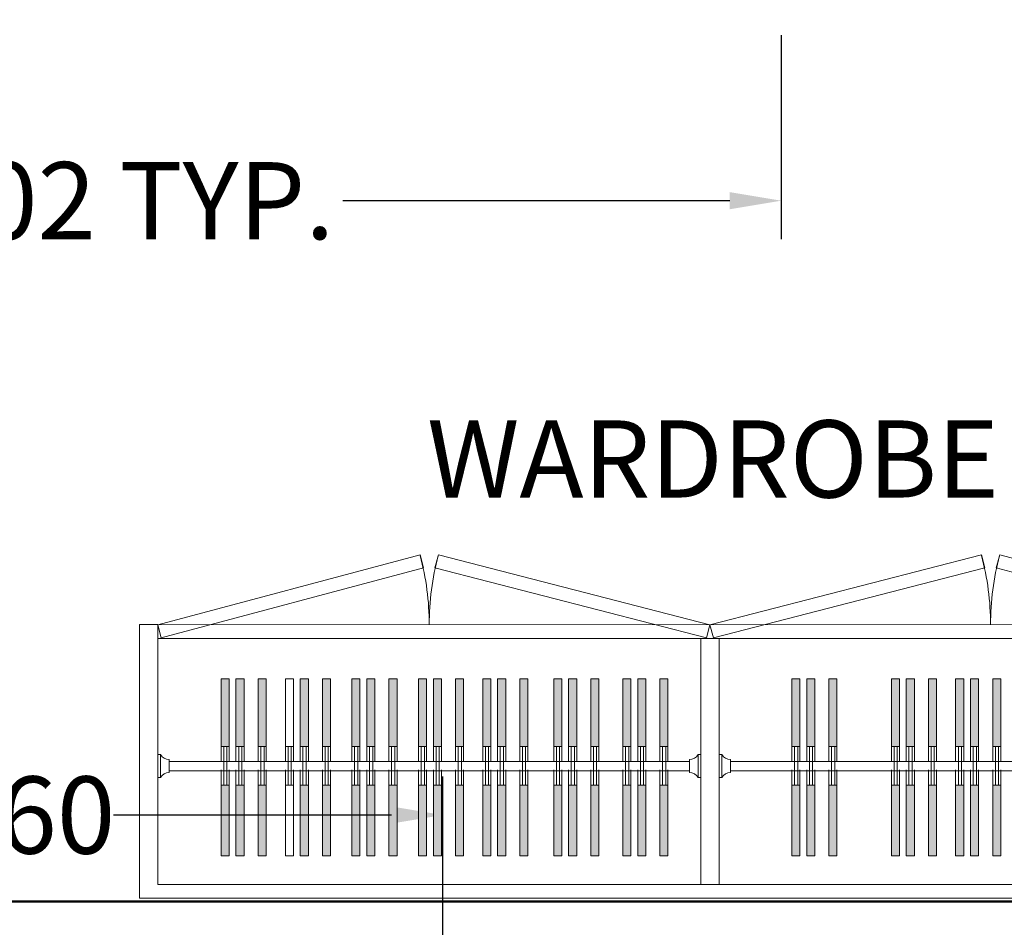
# Model space of a CAD drawing. Units: inches. Extents: x -466983 to 1020, y 324 to 318697.
# Tile 94 of 97: x 864 to 940, y 827 to 898. Entities that reach past the tile are written whole.
import ezdxf

# ---------------------------------------------------------------- set-up
doc = ezdxf.new("R2010")
doc.units = ezdxf.units.IN
doc.header["$MEASUREMENT"] = 0
for name, color, linetype, lineweight in [('A-ANNO-DIMS', 2, 'Continuous', 18), ('A-ANNO-TEXT', 7, 'Continuous', 18), ('A-FLOR-PATT', 252, 'Continuous', 13), ('A-FURN', 8, 'Continuous', 18), ('A-WALL', 7, 'Continuous', 50)]:
    doc.layers.add(name, color=color, linetype=linetype, lineweight=lineweight)
doc.styles.get("Standard").update_dxf_attribs({"font": 'arial.ttf'})
doc.dimstyles.get("Standard").update_dxf_attribs({"dimtxt": 6, "dimasz": 4, "dimexe": 3, "dimexo": 3, "dimgap": 0.09, "dimtad": 0, "dimtih": 1, "dimtoh": 1, "dimdec": 1, "dimzin": 0, "dimdsep": 46, "dimlunit": 3, "dimtxsty": 'Standard', "dimcen": 0.09, "dimadec": 0, "dimazin": 0, "dimtfac": 1, "dimtdec": 1, "dimtofl": 0, "dimtmove": 0, "dimatfit": 3, "dimfxl": 1, "dimtolj": 1, "dimtzin": 0, "dimarcsym": 0})

# ---------------------------------------------------------------- blocks, each defined once
blk = doc.blocks.new('Wardrobe')
h = blk.add_hatch(color=256)
h.dxf.hatch_style = 1
h.paths.add_polyline_path([(2766.949, 1539.754), (2766.159, 1539.754), (2766.159, 1532.86), (2766.949, 1532.86)])
h.paths.add_polyline_path([(2766.949, 1529.069), (2766.159, 1529.069), (2766.159, 1522.476), (2766.949, 1522.476)])
h.paths.add_polyline_path([(2799.415, 1529.068), (2798.626, 1529.068), (2798.626, 1522.475), (2799.415, 1522.475)])
h.paths.add_polyline_path([(2799.415, 1539.753), (2798.626, 1539.753), (2798.626, 1532.859), (2799.415, 1532.859)])
h.paths.add_polyline_path([(2813.081, 1539.753), (2812.292, 1539.753), (2812.292, 1532.859), (2813.081, 1532.859)])
h.paths.add_polyline_path([(2813.081, 1529.068), (2812.292, 1529.068), (2812.292, 1522.475), (2813.081, 1522.475)])
h.paths.add_polyline_path([(2825.842, 1539.753), (2825.053, 1539.753), (2825.053, 1532.859), (2825.842, 1532.859)])
h.paths.add_polyline_path([(2825.842, 1529.068), (2825.053, 1529.068), (2825.053, 1522.475), (2825.842, 1522.475)])
h.paths.add_polyline_path([(2782.932, 1539.754), (2782.143, 1539.754), (2782.143, 1532.86), (2782.932, 1532.86)])
h.paths.add_polyline_path([(2782.932, 1529.069), (2782.143, 1529.069), (2782.143, 1522.476), (2782.932, 1522.476)])
h.paths.add_polyline_path([(2838.604, 1539.753), (2837.814, 1539.753), (2837.814, 1532.859), (2838.604, 1532.859)])
h.paths.add_polyline_path([(2838.604, 1529.068), (2837.814, 1529.068), (2837.814, 1522.475), (2838.604, 1522.475)])
h = blk.add_hatch(color=256)
h.dxf.hatch_style = 1
h.paths.add_polyline_path([(2769.108, 1539.754), (2768.319, 1539.754), (2768.319, 1532.86), (2769.108, 1532.86)])
h.paths.add_polyline_path([(2769.108, 1529.069), (2768.319, 1529.069), (2768.319, 1522.476), (2769.108, 1522.476)])
h.paths.add_polyline_path([(2801.574, 1539.753), (2800.785, 1539.753), (2800.785, 1532.859), (2801.574, 1532.859)])
h.paths.add_polyline_path([(2801.574, 1529.068), (2800.785, 1529.068), (2800.785, 1522.475), (2801.574, 1522.475)])
h.paths.add_polyline_path([(2815.241, 1539.753), (2814.451, 1539.753), (2814.451, 1532.859), (2815.241, 1532.859)])
h.paths.add_polyline_path([(2815.241, 1529.068), (2814.451, 1529.068), (2814.451, 1522.475), (2815.241, 1522.475)])
h.paths.add_polyline_path([(2828.002, 1529.068), (2827.213, 1529.068), (2827.213, 1522.475), (2828.002, 1522.475)])
h.paths.add_polyline_path([(2828.002, 1539.753), (2827.213, 1539.753), (2827.213, 1532.859), (2828.002, 1532.859)])
h.paths.add_polyline_path([(2840.763, 1539.753), (2839.974, 1539.753), (2839.974, 1532.859), (2840.763, 1532.859)])
h.paths.add_polyline_path([(2840.763, 1529.068), (2839.974, 1529.068), (2839.974, 1522.475), (2840.763, 1522.475)])
h.paths.add_polyline_path([(2785.092, 1539.754), (2784.303, 1539.754), (2784.303, 1532.86), (2785.092, 1532.86)])
h.paths.add_polyline_path([(2785.092, 1529.069), (2784.303, 1529.069), (2784.303, 1522.476), (2785.092, 1522.476)])
h = blk.add_hatch(color=256)
h.dxf.hatch_style = 1
h.paths.add_polyline_path([(2770.561, 1539.754), (2769.772, 1539.754), (2769.772, 1532.86), (2770.561, 1532.86)])
h.paths.add_polyline_path([(2770.561, 1529.069), (2769.772, 1529.069), (2769.772, 1522.476), (2770.561, 1522.476)])
h.paths.add_polyline_path([(2786.545, 1539.754), (2785.755, 1539.754), (2785.755, 1532.86), (2786.545, 1532.86)])
h.paths.add_polyline_path([(2786.545, 1529.069), (2785.755, 1529.069), (2785.755, 1522.476), (2786.545, 1522.476)])
h.paths.add_polyline_path([(2803.027, 1539.753), (2802.238, 1539.753), (2802.238, 1532.859), (2803.027, 1532.859)])
h.paths.add_polyline_path([(2803.027, 1529.068), (2802.238, 1529.068), (2802.238, 1522.475), (2803.027, 1522.475)])
h.paths.add_polyline_path([(2816.694, 1539.753), (2815.904, 1539.753), (2815.904, 1532.859), (2816.694, 1532.859)])
h.paths.add_polyline_path([(2816.694, 1529.068), (2815.904, 1529.068), (2815.904, 1522.475), (2816.694, 1522.475)])
h = blk.add_hatch(color=256)
h.dxf.hatch_style = 1
h.paths.add_polyline_path([(2773.218, 1539.754), (2772.429, 1539.754), (2772.429, 1532.86), (2773.218, 1532.86)])
h.paths.add_polyline_path([(2806.159, 1539.753), (2805.37, 1539.753), (2805.37, 1532.859), (2806.159, 1532.859)])
h.paths.add_polyline_path([(2806.159, 1529.068), (2805.37, 1529.068), (2805.37, 1522.475), (2806.159, 1522.475)])
h.paths.add_polyline_path([(2773.218, 1529.069), (2772.429, 1529.069), (2772.429, 1522.476), (2773.218, 1522.476)])
h.paths.add_polyline_path([(2819.351, 1539.753), (2818.562, 1539.753), (2818.562, 1532.859), (2819.351, 1532.859)])
h.paths.add_polyline_path([(2819.351, 1529.068), (2818.562, 1529.068), (2818.562, 1522.475), (2819.351, 1522.475)])
h.paths.add_polyline_path([(2832.334, 1539.753), (2831.545, 1539.753), (2831.545, 1532.859), (2832.334, 1532.859)])
h.paths.add_polyline_path([(2832.334, 1529.068), (2831.545, 1529.068), (2831.545, 1522.475), (2832.334, 1522.475)])
h = blk.add_hatch(color=256)
h.dxf.hatch_style = 1
h.paths.add_polyline_path([(2775.378, 1539.754), (2774.589, 1539.754), (2774.589, 1532.86), (2775.378, 1532.86)])
h.paths.add_polyline_path([(2775.378, 1529.069), (2774.589, 1529.069), (2774.589, 1522.476), (2775.378, 1522.476)])
h.paths.add_polyline_path([(2808.319, 1539.753), (2807.529, 1539.753), (2807.529, 1532.859), (2808.319, 1532.859)])
h.paths.add_polyline_path([(2808.319, 1529.068), (2807.529, 1529.068), (2807.529, 1522.475), (2808.319, 1522.475)])
h.paths.add_polyline_path([(2834.494, 1539.753), (2833.704, 1539.753), (2833.704, 1532.859), (2834.494, 1532.859)])
h.paths.add_polyline_path([(2834.494, 1529.068), (2833.704, 1529.068), (2833.704, 1522.475), (2834.494, 1522.475)])
h = blk.add_hatch(color=256)
h.dxf.hatch_style = 1
h.paths.add_polyline_path([(2776.831, 1539.754), (2776.041, 1539.754), (2776.041, 1532.86), (2776.831, 1532.86)])
h.paths.add_polyline_path([(2776.831, 1529.069), (2776.041, 1529.069), (2776.041, 1522.476), (2776.831, 1522.476)])
h.paths.add_polyline_path([(2809.772, 1539.753), (2808.982, 1539.753), (2808.982, 1532.859), (2809.772, 1532.859)])
h.paths.add_polyline_path([(2809.772, 1529.068), (2808.982, 1529.068), (2808.982, 1522.475), (2809.772, 1522.475)])
h.paths.add_polyline_path([(2821.51, 1539.753), (2820.721, 1539.753), (2820.721, 1532.859), (2821.51, 1532.859)])
h.paths.add_polyline_path([(2821.51, 1529.068), (2820.721, 1529.068), (2820.721, 1522.475), (2821.51, 1522.475)])
h = blk.add_hatch(color=256)
h.dxf.hatch_style = 1
h.paths.add_polyline_path([(2822.963, 1539.753), (2822.174, 1539.753), (2822.174, 1532.859), (2822.963, 1532.859)])
h.paths.add_polyline_path([(2822.963, 1529.068), (2822.174, 1529.068), (2822.174, 1522.475), (2822.963, 1522.475)])
h = blk.add_hatch(color=256)
h.dxf.hatch_style = 1
h.paths.add_polyline_path([(2829.455, 1539.753), (2828.665, 1539.753), (2828.665, 1532.859), (2829.455, 1532.859)])
h.paths.add_polyline_path([(2829.455, 1529.068), (2828.665, 1529.068), (2828.665, 1522.475), (2829.455, 1522.475)])
h.paths.add_polyline_path([(2842.216, 1539.753), (2841.427, 1539.753), (2841.427, 1532.859), (2842.216, 1532.859)])
h.paths.add_polyline_path([(2842.216, 1529.068), (2841.427, 1529.068), (2841.427, 1522.475), (2842.216, 1522.475)])
for p, q in [((2738.889, 1517.193, 0), (2738.889, 1543.902, 0)), ((2738.889, 1543.902, 0), (2850.181, 1543.902, 0)), ((2850.181, 1543.902, 0), (2850.181, 1517.191, 0)), ((2848.4, 1542.566, 0), (2740.67, 1542.566, 0)), ((2740.67, 1542.566, 0), (2740.67, 1517.193, 0)), ((2793.645, 1542.566, 0), (2793.645, 1518.528, 0)), ((2795.425, 1542.566, 0), (2795.425, 1518.528, 0)), ((2848.4, 1517.191, 0), (2848.4, 1542.566, 0)), ((2740.937, 1532.105, 0), (2740.67, 1532.105, 0)), ((2740.937, 1532.105, 0), (2740.67, 1532.105, 0)), ((2740.937, 1532.105, 0), (2740.937, 1529.879, 0)), ((2740.937, 1532.105, 0), (2740.937, 1529.879, 0)), ((2793.377, 1532.105, 0), (2793.377, 1529.879, 0)), ((2793.377, 1532.105, 0), (2793.377, 1529.879, 0)), ((2793.377, 1532.105, 0), (2793.645, 1532.105, 0)), ((2793.377, 1532.105, 0), (2793.645, 1532.105, 0)), ((2795.692, 1532.105, 0), (2795.425, 1532.105, 0)), ((2795.692, 1532.105, 0), (2795.425, 1532.105, 0)), ((2795.692, 1532.105, 0), (2795.692, 1529.879, 0)), ((2795.692, 1532.105, 0), (2795.692, 1529.879, 0)), ((2848.133, 1532.105, 0), (2848.133, 1529.879, 0)), ((2848.133, 1532.105, 0), (2848.133, 1529.879, 0)), ((2848.133, 1532.105, 0), (2848.4, 1532.105, 0)), ((2848.133, 1532.105, 0), (2848.4, 1532.105, 0)), ((2741.783, 1531.615, 0), (2741.783, 1530.369, 0)), ((2741.783, 1531.453, 0), (2792.532, 1531.453, 0)), ((2792.532, 1531.615, 0), (2792.532, 1530.369, 0)), ((2796.538, 1531.615, 0), (2796.538, 1530.369, 0)), ((2796.538, 1531.453, 0), (2847.287, 1531.453, 0)), ((2847.287, 1531.615, 0), (2847.287, 1530.369, 0)), ((2741.783, 1530.563, 0), (2792.532, 1530.563, 0)), ((2796.538, 1530.563, 0), (2847.287, 1530.563, 0)), ((2740.937, 1529.879, 0), (2740.67, 1529.879, 0)), ((2740.937, 1529.879, 0), (2740.67, 1529.879, 0)), ((2793.377, 1529.879, 0), (2793.645, 1529.879, 0)), ((2793.377, 1529.879, 0), (2793.645, 1529.879, 0)), ((2795.692, 1529.879, 0), (2795.425, 1529.879, 0)), ((2795.692, 1529.879, 0), (2795.425, 1529.879, 0)), ((2848.133, 1529.879, 0), (2848.4, 1529.879, 0)), ((2848.133, 1529.879, 0), (2848.4, 1529.879, 0)), ((2848.4, 1518.527, 0), (2740.67, 1518.528, 0)), ((2795.425, 1518.528, 0), (2793.645, 1518.528, 0)), ((2740.67, 1517.192, 0), (2741.015, 1518.481, 0)), ((2741.015, 1518.481, 0), (2766.604, 1511.655, 0)), ((2794.189, 1518.481, 0), (2767.71, 1511.655, 0)), ((2794.535, 1517.192, 0), (2794.189, 1518.481, 0)), ((2794.535, 1517.192, 0), (2794.88, 1518.481, 0)), ((2794.88, 1518.481, 0), (2821.359, 1511.655, 0)), ((2848.054, 1518.481, 0), (2822.466, 1511.655, 0)), ((2848.4, 1517.192, 0), (2848.054, 1518.481, 0)), ((2740.67, 1517.193, 0), (2738.889, 1517.193, 0)), ((2848.4, 1517.191, 0), (2740.67, 1517.193, 0)), ((2766.258, 1510.365, 0), (2740.67, 1517.192, 0)), ((2768.056, 1510.365, 0), (2794.535, 1517.192, 0)), ((2821.014, 1510.365, 0), (2794.535, 1517.192, 0)), ((2822.811, 1510.365, 0), (2848.4, 1517.192, 0)), ((2850.181, 1517.191, 0), (2848.4, 1517.191, 0)), ((2766.604, 1511.655, 0), (2766.258, 1510.365, 0)), ((2767.71, 1511.655, 0), (2768.056, 1510.365, 0)), ((2821.359, 1511.655, 0), (2821.014, 1510.365, 0)), ((2822.466, 1511.655, 0), (2822.811, 1510.365, 0))]:
    blk.add_line(p, q)
at = {"ltscale": 0.106667}
for p, q in [((2745.324, 1522.089, 0), (2763.131, 1539.896, 0)), ((2745.324, 1522.089, 0), (2745.324, 1539.896, 0)), ((2745.324, 1539.896, 0), (2763.131, 1539.896, 0)), ((2763.131, 1522.089, 0), (2745.324, 1539.896, 0)), ((2763.131, 1539.896, 0), (2763.131, 1522.089, 0)), ((2763.131, 1522.089, 0), (2745.324, 1522.089, 0))]:
    blk.add_line(p, q, dxfattribs=at)
at = {"ltscale": 0.037333}
for p, q in [((2766.159, 1531.365, 0), (2766.159, 1539.754, 0)), ((2766.159, 1539.754, 0), (2766.949, 1539.754, 0)), ((2766.949, 1539.754, 0), (2766.949, 1531.365, 0)), ((2768.319, 1531.365, 0), (2768.319, 1539.754, 0)), ((2768.319, 1539.754, 0), (2769.108, 1539.754, 0)), ((2769.108, 1539.754, 0), (2769.108, 1531.365, 0)), ((2769.772, 1531.365, 0), (2769.772, 1539.754, 0)), ((2769.772, 1539.754, 0), (2770.561, 1539.754, 0)), ((2770.561, 1539.754, 0), (2770.561, 1531.365, 0)), ((2772.429, 1531.365, 0), (2772.429, 1539.754, 0)), ((2772.429, 1539.754, 0), (2773.218, 1539.754, 0)), ((2773.218, 1539.754, 0), (2773.218, 1531.365, 0)), ((2774.589, 1531.365, 0), (2774.589, 1539.754, 0)), ((2774.589, 1539.754, 0), (2775.378, 1539.754, 0)), ((2775.378, 1539.754, 0), (2775.378, 1531.365, 0)), ((2776.041, 1531.365, 0), (2776.041, 1539.754, 0)), ((2776.041, 1539.754, 0), (2776.831, 1539.754, 0)), ((2776.831, 1539.754, 0), (2776.831, 1531.365, 0)), ((2782.143, 1531.365, 0), (2782.143, 1539.754, 0)), ((2782.143, 1539.754, 0), (2782.932, 1539.754, 0)), ((2782.932, 1539.754, 0), (2782.932, 1531.365, 0)), ((2784.303, 1531.365, 0), (2784.303, 1539.754, 0)), ((2784.303, 1539.754, 0), (2785.092, 1539.754, 0)), ((2785.092, 1539.754, 0), (2785.092, 1531.365, 0)), ((2785.755, 1531.365, 0), (2785.755, 1539.754, 0)), ((2785.755, 1539.754, 0), (2786.545, 1539.754, 0)), ((2786.545, 1539.754, 0), (2786.545, 1531.365, 0)), ((2798.626, 1531.364, 0), (2798.626, 1539.753, 0)), ((2798.626, 1539.753, 0), (2799.415, 1539.753, 0)), ((2799.415, 1539.753, 0), (2799.415, 1531.364, 0)), ((2800.785, 1531.364, 0), (2800.785, 1539.753, 0)), ((2800.785, 1539.753, 0), (2801.574, 1539.753, 0)), ((2801.574, 1539.753, 0), (2801.574, 1531.364, 0)), ((2802.238, 1531.364, 0), (2802.238, 1539.753, 0)), ((2802.238, 1539.753, 0), (2803.027, 1539.753, 0)), ((2803.027, 1539.753, 0), (2803.027, 1531.364, 0)), ((2805.37, 1531.364, 0), (2805.37, 1539.753, 0)), ((2805.37, 1539.753, 0), (2806.159, 1539.753, 0)), ((2806.159, 1539.753, 0), (2806.159, 1531.364, 0)), ((2807.529, 1531.364, 0), (2807.529, 1539.753, 0)), ((2807.529, 1539.753, 0), (2808.319, 1539.753, 0)), ((2808.319, 1539.753, 0), (2808.319, 1531.364, 0)), ((2808.982, 1531.364, 0), (2808.982, 1539.753, 0)), ((2808.982, 1539.753, 0), (2809.772, 1539.753, 0)), ((2809.772, 1539.753, 0), (2809.772, 1531.364, 0)), ((2812.292, 1531.364, 0), (2812.292, 1539.753, 0)), ((2812.292, 1539.753, 0), (2813.081, 1539.753, 0)), ((2813.081, 1539.753, 0), (2813.081, 1531.364, 0)), ((2814.451, 1531.364, 0), (2814.451, 1539.753, 0)), ((2814.451, 1539.753, 0), (2815.241, 1539.753, 0)), ((2815.241, 1539.753, 0), (2815.241, 1531.364, 0)), ((2815.904, 1531.364, 0), (2815.904, 1539.753, 0)), ((2815.904, 1539.753, 0), (2816.694, 1539.753, 0)), ((2816.694, 1539.753, 0), (2816.694, 1531.364, 0)), ((2818.562, 1531.364, 0), (2818.562, 1539.753, 0)), ((2818.562, 1539.753, 0), (2819.351, 1539.753, 0)), ((2819.351, 1539.753, 0), (2819.351, 1531.364, 0)), ((2820.721, 1531.364, 0), (2820.721, 1539.753, 0)), ((2820.721, 1539.753, 0), (2821.51, 1539.753, 0)), ((2821.51, 1539.753, 0), (2821.51, 1531.364, 0)), ((2822.174, 1531.364, 0), (2822.174, 1539.753, 0)), ((2822.174, 1539.753, 0), (2822.963, 1539.753, 0)), ((2822.963, 1539.753, 0), (2822.963, 1531.364, 0)), ((2825.053, 1531.364, 0), (2825.053, 1539.753, 0)), ((2825.053, 1539.753, 0), (2825.842, 1539.753, 0)), ((2825.842, 1539.753, 0), (2825.842, 1531.364, 0)), ((2827.213, 1531.364, 0), (2827.213, 1539.753, 0)), ((2827.213, 1539.753, 0), (2828.002, 1539.753, 0)), ((2828.002, 1539.753, 0), (2828.002, 1531.364, 0)), ((2828.665, 1531.364, 0), (2828.665, 1539.753, 0)), ((2828.665, 1539.753, 0), (2829.455, 1539.753, 0)), ((2829.455, 1539.753, 0), (2829.455, 1531.364, 0)), ((2831.545, 1531.364, 0), (2831.545, 1539.753, 0)), ((2831.545, 1539.753, 0), (2832.334, 1539.753, 0)), ((2832.334, 1539.753, 0), (2832.334, 1531.364, 0)), ((2833.704, 1531.364, 0), (2833.704, 1539.753, 0)), ((2833.704, 1539.753, 0), (2834.494, 1539.753, 0)), ((2834.494, 1539.753, 0), (2834.494, 1531.364, 0)), ((2835.157, 1531.364, 0), (2835.157, 1539.753, 0)), ((2835.157, 1539.753, 0), (2835.946, 1539.753, 0)), ((2835.946, 1539.753, 0), (2835.946, 1531.364, 0)), ((2837.814, 1531.364, 0), (2837.814, 1539.753, 0)), ((2837.814, 1539.753, 0), (2838.604, 1539.753, 0)), ((2838.604, 1539.753, 0), (2838.604, 1531.364, 0)), ((2839.974, 1531.364, 0), (2839.974, 1539.753, 0)), ((2839.974, 1539.753, 0), (2840.763, 1539.753, 0)), ((2840.763, 1539.753, 0), (2840.763, 1531.364, 0)), ((2841.427, 1531.364, 0), (2841.427, 1539.753, 0)), ((2841.427, 1539.753, 0), (2842.216, 1539.753, 0)), ((2842.216, 1539.753, 0), (2842.216, 1531.364, 0)), ((2766.159, 1532.86, 0), (2766.949, 1532.86, 0)), ((2766.373, 1529.069, 0), (2766.373, 1532.86, 0)), ((2766.685, 1529.069, 0), (2766.685, 1532.86, 0)), ((2768.319, 1532.86, 0), (2769.108, 1532.86, 0)), ((2768.533, 1529.069, 0), (2768.533, 1532.86, 0)), ((2768.845, 1529.069, 0), (2768.845, 1532.86, 0)), ((2769.772, 1532.86, 0), (2770.561, 1532.86, 0)), ((2769.986, 1529.069, 0), (2769.986, 1532.86, 0)), ((2770.298, 1529.069, 0), (2770.298, 1532.86, 0)), ((2772.429, 1532.86, 0), (2773.218, 1532.86, 0)), ((2772.643, 1529.069, 0), (2772.643, 1532.86, 0)), ((2772.955, 1529.069, 0), (2772.955, 1532.86, 0)), ((2774.589, 1532.86, 0), (2775.378, 1532.86, 0)), ((2774.803, 1529.069, 0), (2774.803, 1532.86, 0)), ((2775.115, 1529.069, 0), (2775.115, 1532.86, 0)), ((2776.041, 1532.86, 0), (2776.831, 1532.86, 0)), ((2776.256, 1529.069, 0), (2776.256, 1532.86, 0)), ((2776.567, 1529.069, 0), (2776.567, 1532.86, 0)), ((2782.143, 1532.86, 0), (2782.932, 1532.86, 0)), ((2782.357, 1529.069, 0), (2782.357, 1532.86, 0)), ((2782.669, 1529.069, 0), (2782.669, 1532.86, 0)), ((2784.303, 1532.86, 0), (2785.092, 1532.86, 0)), ((2784.517, 1529.069, 0), (2784.517, 1532.86, 0)), ((2784.829, 1529.069, 0), (2784.829, 1532.86, 0)), ((2785.755, 1532.86, 0), (2786.545, 1532.86, 0)), ((2785.969, 1529.069, 0), (2785.969, 1532.86, 0)), ((2786.281, 1529.069, 0), (2786.281, 1532.86, 0)), ((2798.626, 1532.859, 0), (2799.415, 1532.859, 0)), ((2798.84, 1529.068, 0), (2798.84, 1532.859, 0)), ((2799.152, 1529.068, 0), (2799.152, 1532.859, 0)), ((2800.785, 1532.859, 0), (2801.574, 1532.859, 0)), ((2800.999, 1529.068, 0), (2800.999, 1532.859, 0)), ((2801.311, 1529.068, 0), (2801.311, 1532.859, 0)), ((2802.238, 1532.859, 0), (2803.027, 1532.859, 0)), ((2802.452, 1529.068, 0), (2802.452, 1532.859, 0)), ((2802.764, 1529.068, 0), (2802.764, 1532.859, 0)), ((2805.37, 1532.859, 0), (2806.159, 1532.859, 0)), ((2805.584, 1529.068, 0), (2805.584, 1532.859, 0)), ((2805.896, 1529.068, 0), (2805.896, 1532.859, 0)), ((2807.529, 1532.859, 0), (2808.319, 1532.859, 0)), ((2807.744, 1529.068, 0), (2807.744, 1532.859, 0)), ((2808.056, 1529.068, 0), (2808.056, 1532.859, 0)), ((2808.982, 1532.859, 0), (2809.772, 1532.859, 0)), ((2809.196, 1529.068, 0), (2809.196, 1532.859, 0)), ((2809.508, 1529.068, 0), (2809.508, 1532.859, 0)), ((2812.292, 1532.859, 0), (2813.081, 1532.859, 0)), ((2812.506, 1529.068, 0), (2812.506, 1532.859, 0)), ((2812.818, 1529.068, 0), (2812.818, 1532.859, 0)), ((2814.451, 1532.859, 0), (2815.241, 1532.859, 0)), ((2814.665, 1529.068, 0), (2814.665, 1532.859, 0)), ((2814.977, 1529.068, 0), (2814.977, 1532.859, 0)), ((2815.904, 1532.859, 0), (2816.694, 1532.859, 0)), ((2816.118, 1529.068, 0), (2816.118, 1532.859, 0)), ((2816.43, 1529.068, 0), (2816.43, 1532.859, 0)), ((2818.562, 1532.859, 0), (2819.351, 1532.859, 0)), ((2818.776, 1529.068, 0), (2818.776, 1532.859, 0)), ((2819.088, 1529.068, 0), (2819.088, 1532.859, 0)), ((2820.721, 1532.859, 0), (2821.51, 1532.859, 0)), ((2820.935, 1529.068, 0), (2820.935, 1532.859, 0)), ((2821.247, 1529.068, 0), (2821.247, 1532.859, 0)), ((2822.174, 1532.859, 0), (2822.963, 1532.859, 0)), ((2822.388, 1529.068, 0), (2822.388, 1532.859, 0)), ((2822.7, 1529.068, 0), (2822.7, 1532.859, 0)), ((2825.053, 1532.859, 0), (2825.842, 1532.859, 0)), ((2825.267, 1529.068, 0), (2825.267, 1532.859, 0)), ((2825.579, 1529.068, 0), (2825.579, 1532.859, 0)), ((2827.213, 1532.859, 0), (2828.002, 1532.859, 0)), ((2827.427, 1529.068, 0), (2827.427, 1532.859, 0)), ((2827.739, 1529.068, 0), (2827.739, 1532.859, 0)), ((2828.665, 1532.859, 0), (2829.455, 1532.859, 0)), ((2828.88, 1529.068, 0), (2828.88, 1532.859, 0)), ((2829.191, 1529.068, 0), (2829.191, 1532.859, 0)), ((2831.545, 1532.859, 0), (2832.334, 1532.859, 0)), ((2831.759, 1529.068, 0), (2831.759, 1532.859, 0)), ((2832.071, 1529.068, 0), (2832.071, 1532.859, 0)), ((2833.704, 1532.859, 0), (2834.494, 1532.859, 0)), ((2833.918, 1529.068, 0), (2833.918, 1532.859, 0)), ((2834.23, 1529.068, 0), (2834.23, 1532.859, 0)), ((2835.157, 1532.859, 0), (2835.946, 1532.859, 0)), ((2835.371, 1529.068, 0), (2835.371, 1532.859, 0)), ((2835.683, 1529.068, 0), (2835.683, 1532.859, 0)), ((2837.814, 1532.859, 0), (2838.604, 1532.859, 0)), ((2838.028, 1529.068, 0), (2838.028, 1532.859, 0)), ((2838.34, 1529.068, 0), (2838.34, 1532.859, 0)), ((2839.974, 1532.859, 0), (2840.763, 1532.859, 0)), ((2840.188, 1529.068, 0), (2840.188, 1532.859, 0)), ((2840.5, 1529.068, 0), (2840.5, 1532.859, 0)), ((2841.427, 1532.859, 0), (2842.216, 1532.859, 0)), ((2841.641, 1529.068, 0), (2841.641, 1532.859, 0)), ((2841.953, 1529.068, 0), (2841.953, 1532.859, 0)), ((2766.159, 1522.476, 0), (2766.159, 1530.564, 0)), ((2766.949, 1530.564, 0), (2766.949, 1522.476, 0)), ((2768.319, 1522.476, 0), (2768.319, 1530.564, 0)), ((2769.108, 1530.564, 0), (2769.108, 1522.476, 0)), ((2769.772, 1522.476, 0), (2769.772, 1530.564, 0)), ((2770.561, 1530.564, 0), (2770.561, 1522.476, 0)), ((2772.429, 1522.476, 0), (2772.429, 1530.564, 0)), ((2773.218, 1530.564, 0), (2773.218, 1522.476, 0)), ((2774.589, 1522.476, 0), (2774.589, 1530.564, 0)), ((2775.378, 1530.564, 0), (2775.378, 1522.476, 0)), ((2776.041, 1522.476, 0), (2776.041, 1530.564, 0)), ((2776.831, 1530.564, 0), (2776.831, 1522.476, 0)), ((2782.143, 1522.476, 0), (2782.143, 1530.564, 0)), ((2782.932, 1530.564, 0), (2782.932, 1522.476, 0)), ((2784.303, 1522.476, 0), (2784.303, 1530.564, 0)), ((2785.092, 1530.564, 0), (2785.092, 1522.476, 0)), ((2785.755, 1522.476, 0), (2785.755, 1530.564, 0)), ((2786.545, 1530.564, 0), (2786.545, 1522.476, 0)), ((2798.626, 1522.475, 0), (2798.626, 1530.563, 0)), ((2799.415, 1530.563, 0), (2799.415, 1522.475, 0)), ((2800.785, 1522.475, 0), (2800.785, 1530.563, 0)), ((2801.574, 1530.563, 0), (2801.574, 1522.475, 0)), ((2802.238, 1522.475, 0), (2802.238, 1530.563, 0)), ((2803.027, 1530.563, 0), (2803.027, 1522.475, 0)), ((2805.37, 1522.475, 0), (2805.37, 1530.563, 0)), ((2806.159, 1530.563, 0), (2806.159, 1522.475, 0)), ((2807.529, 1522.475, 0), (2807.529, 1530.563, 0)), ((2808.319, 1530.563, 0), (2808.319, 1522.475, 0)), ((2808.982, 1522.475, 0), (2808.982, 1530.563, 0)), ((2809.772, 1530.563, 0), (2809.772, 1522.475, 0)), ((2812.292, 1522.475, 0), (2812.292, 1530.563, 0)), ((2813.081, 1530.563, 0), (2813.081, 1522.475, 0)), ((2814.451, 1522.475, 0), (2814.451, 1530.563, 0)), ((2815.241, 1530.563, 0), (2815.241, 1522.475, 0)), ((2815.904, 1522.475, 0), (2815.904, 1530.563, 0)), ((2816.694, 1530.563, 0), (2816.694, 1522.475, 0)), ((2818.562, 1522.475, 0), (2818.562, 1530.563, 0)), ((2819.351, 1530.563, 0), (2819.351, 1522.475, 0)), ((2820.721, 1522.475, 0), (2820.721, 1530.563, 0)), ((2821.51, 1530.563, 0), (2821.51, 1522.475, 0)), ((2822.174, 1522.475, 0), (2822.174, 1530.563, 0)), ((2822.963, 1530.563, 0), (2822.963, 1522.475, 0)), ((2825.053, 1522.475, 0), (2825.053, 1530.563, 0)), ((2825.842, 1530.563, 0), (2825.842, 1522.475, 0)), ((2827.213, 1522.475, 0), (2827.213, 1530.563, 0)), ((2828.002, 1530.563, 0), (2828.002, 1522.475, 0)), ((2828.665, 1522.475, 0), (2828.665, 1530.563, 0)), ((2829.455, 1530.563, 0), (2829.455, 1522.475, 0)), ((2831.545, 1522.475, 0), (2831.545, 1530.563, 0)), ((2832.334, 1530.563, 0), (2832.334, 1522.475, 0)), ((2833.704, 1522.475, 0), (2833.704, 1530.563, 0)), ((2834.494, 1530.563, 0), (2834.494, 1522.475, 0)), ((2835.157, 1522.475, 0), (2835.157, 1530.563, 0)), ((2835.946, 1530.563, 0), (2835.946, 1522.475, 0)), ((2837.814, 1522.475, 0), (2837.814, 1530.563, 0)), ((2838.604, 1530.563, 0), (2838.604, 1522.475, 0)), ((2839.974, 1522.475, 0), (2839.974, 1530.563, 0)), ((2840.763, 1530.563, 0), (2840.763, 1522.475, 0)), ((2841.427, 1522.475, 0), (2841.427, 1530.563, 0)), ((2842.216, 1530.563, 0), (2842.216, 1522.475, 0)), ((2766.159, 1529.069, 0), (2766.949, 1529.069, 0)), ((2768.319, 1529.069, 0), (2769.108, 1529.069, 0)), ((2769.772, 1529.069, 0), (2770.561, 1529.069, 0)), ((2772.429, 1529.069, 0), (2773.218, 1529.069, 0)), ((2774.589, 1529.069, 0), (2775.378, 1529.069, 0)), ((2776.041, 1529.069, 0), (2776.831, 1529.069, 0)), ((2782.143, 1529.069, 0), (2782.932, 1529.069, 0)), ((2784.303, 1529.069, 0), (2785.092, 1529.069, 0)), ((2785.755, 1529.069, 0), (2786.545, 1529.069, 0)), ((2798.626, 1529.068, 0), (2799.415, 1529.068, 0)), ((2800.785, 1529.068, 0), (2801.574, 1529.068, 0)), ((2802.238, 1529.068, 0), (2803.027, 1529.068, 0)), ((2805.37, 1529.068, 0), (2806.159, 1529.068, 0)), ((2807.529, 1529.068, 0), (2808.319, 1529.068, 0)), ((2808.982, 1529.068, 0), (2809.772, 1529.068, 0)), ((2812.292, 1529.068, 0), (2813.081, 1529.068, 0)), ((2814.451, 1529.068, 0), (2815.241, 1529.068, 0)), ((2815.904, 1529.068, 0), (2816.694, 1529.068, 0)), ((2818.562, 1529.068, 0), (2819.351, 1529.068, 0)), ((2820.721, 1529.068, 0), (2821.51, 1529.068, 0)), ((2822.174, 1529.068, 0), (2822.963, 1529.068, 0)), ((2825.053, 1529.068, 0), (2825.842, 1529.068, 0)), ((2827.213, 1529.068, 0), (2828.002, 1529.068, 0)), ((2828.665, 1529.068, 0), (2829.455, 1529.068, 0)), ((2831.545, 1529.068, 0), (2832.334, 1529.068, 0)), ((2833.704, 1529.068, 0), (2834.494, 1529.068, 0)), ((2835.157, 1529.068, 0), (2835.946, 1529.068, 0)), ((2837.814, 1529.068, 0), (2838.604, 1529.068, 0)), ((2839.974, 1529.068, 0), (2840.763, 1529.068, 0)), ((2841.427, 1529.068, 0), (2842.216, 1529.068, 0)), ((2766.949, 1522.476, 0), (2766.159, 1522.476, 0)), ((2769.108, 1522.476, 0), (2768.319, 1522.476, 0)), ((2770.561, 1522.476, 0), (2769.772, 1522.476, 0)), ((2773.218, 1522.476, 0), (2772.429, 1522.476, 0)), ((2775.378, 1522.476, 0), (2774.589, 1522.476, 0)), ((2776.831, 1522.476, 0), (2776.041, 1522.476, 0)), ((2782.932, 1522.476, 0), (2782.143, 1522.476, 0)), ((2785.092, 1522.476, 0), (2784.303, 1522.476, 0)), ((2786.545, 1522.476, 0), (2785.755, 1522.476, 0)), ((2799.415, 1522.475, 0), (2798.626, 1522.475, 0)), ((2801.574, 1522.475, 0), (2800.785, 1522.475, 0)), ((2803.027, 1522.475, 0), (2802.238, 1522.475, 0)), ((2806.159, 1522.475, 0), (2805.37, 1522.475, 0)), ((2808.319, 1522.475, 0), (2807.529, 1522.475, 0)), ((2809.772, 1522.475, 0), (2808.982, 1522.475, 0)), ((2813.081, 1522.475, 0), (2812.292, 1522.475, 0)), ((2815.241, 1522.475, 0), (2814.451, 1522.475, 0)), ((2816.694, 1522.475, 0), (2815.904, 1522.475, 0)), ((2819.351, 1522.475, 0), (2818.562, 1522.475, 0)), ((2821.51, 1522.475, 0), (2820.721, 1522.475, 0)), ((2822.963, 1522.475, 0), (2822.174, 1522.475, 0)), ((2825.842, 1522.475, 0), (2825.053, 1522.475, 0)), ((2828.002, 1522.475, 0), (2827.213, 1522.475, 0)), ((2829.455, 1522.475, 0), (2828.665, 1522.475, 0)), ((2832.334, 1522.475, 0), (2831.545, 1522.475, 0)), ((2834.494, 1522.475, 0), (2833.704, 1522.475, 0)), ((2835.946, 1522.475, 0), (2835.157, 1522.475, 0)), ((2838.604, 1522.475, 0), (2837.814, 1522.475, 0)), ((2840.763, 1522.475, 0), (2839.974, 1522.475, 0)), ((2842.216, 1522.475, 0), (2841.427, 1522.475, 0))]:
    blk.add_line(p, q, dxfattribs=at)
at = {"ltscale": 0.02}
for p, q in [((2742.337, 1537.369, 0), (2742.843, 1537.497, 0)), ((2742.337, 1534.917, 0), (2742.337, 1537.369, 0)), ((2743.675, 1536.85, 0), (2743.675, 1525.184, 0)), ((2740.67, 1534.917, 0), (2742.845, 1534.917, 0)), ((2740.874, 1534.917, 0), (2740.874, 1535.616, 0)), ((2741.987, 1535.616, 0), (2741.987, 1534.917, 0)), ((2742.845, 1534.917, 0), (2742.845, 1534.532, 0)), ((2742.845, 1534.532, 0), (2740.67, 1534.532, 0)), ((2740.874, 1527.454, 0), (2740.874, 1534.532, 0)), ((2741.987, 1534.532, 0), (2741.987, 1527.454, 0)), ((2742.337, 1527.454, 0), (2742.337, 1534.532, 0)), ((2742.845, 1527.454, 0), (2740.67, 1527.454, 0)), ((2742.845, 1527.068, 0), (2742.845, 1527.454, 0)), ((2740.67, 1527.068, 0), (2742.845, 1527.068, 0)), ((2740.874, 1526.336, 0), (2740.874, 1527.068, 0)), ((2741.987, 1527.068, 0), (2741.987, 1526.336, 0)), ((2742.337, 1524.648, 0), (2742.337, 1527.068, 0)), ((2742.863, 1524.532, 0), (2742.337, 1524.648, 0))]:
    blk.add_line(p, q, dxfattribs=at)
for centre, radius, start, end in [((2743.007, 1536.85, 0), 0.668, 360, 104.18866), ((2741.43, 1535.616, 0), 0.556, 0, 180), ((2741.43, 1526.336, 0), 0.556, 180, 0), ((2743.007, 1525.184, 0), 0.668, 257.52566, 0)]:
    blk.add_arc(centre, radius, start, end, dxfattribs=at)
for centre, radius, start, end in [((2741.784, 1532.592, 0), 0.977, 209.91557, 269.94727), ((2741.784, 1532.592, 0), 0.977, 209.91557, 269.94727), ((2792.531, 1532.592, 0), 0.977, 270.05273, 330.08443), ((2792.531, 1532.592, 0), 0.977, 270.05273, 330.08443), ((2796.539, 1532.592, 0), 0.977, 209.91557, 269.94727), ((2796.539, 1532.592, 0), 0.977, 209.91557, 269.94727), ((2847.286, 1532.592, 0), 0.977, 270.05273, 330.08443), ((2847.286, 1532.592, 0), 0.977, 270.05273, 330.08443), ((2741.784, 1529.392, 0), 0.977, 90.05273, 150.08443), ((2792.531, 1529.392, 0), 0.977, 29.91557, 89.94727), ((2796.539, 1529.392, 0), 0.977, 90.05273, 150.08443), ((2847.286, 1529.392, 0), 0.977, 29.91557, 89.94727), ((2740.781, 1517.191, 0), 26.376, 345.18907, 0), ((2793.533, 1517.191, 0), 26.376, 180, 194.81093), ((2795.537, 1517.192, 0), 26.376, 345.18907, 0), ((2848.289, 1517.192, 0), 26.376, 180, 194.81093)]:
    blk.add_arc(centre, radius, start, end)
blk = doc.blocks.new('*D74')
at = {"layer": 'A-ANNO-DIMS', "color": 0, "lineweight": -2, "transparency": 16777216}
for p, q in [((821.534, 896.315), (821.534, 880.453)), ((923.134, 896.315), (923.134, 880.453)), ((825.534, 883.453), (855.592, 883.453)), ((919.134, 883.453), (889.075, 883.453))]:
    blk.add_line(p, q, dxfattribs=at)
at = {"layer": 'A-ANNO-DIMS', "color": 0, "transparency": 16777216}
for points in [[(825.534, 884.119), (825.534, 882.786), (821.534, 883.453)], [(919.134, 884.119), (919.134, 882.786), (923.134, 883.453)]]:
    blk.add_solid(points, dxfattribs=at)
at = {"layer": 'Defpoints', "color": 0, "transparency": 16777216}
for p in [(821.534, 899.315), (923.134, 899.315), (923.134, 883.453)]:
    blk.add_point(p, dxfattribs=at)
at = {"layer": 'A-ANNO-DIMS', "color": 0, "transparency": 16777216, "insert": (872.334, 883.453), "char_height": 6, "attachment_point": 5}
blk.add_mtext('\\A1;102 TYP.', dxfattribs=at)
blk = doc.blocks.new('*D81')
at = {"layer": 'A-ANNO-DIMS', "color": 0, "lineweight": -2, "transparency": 16777216}
for p, q in [((873.257, 826.195), (873.257, 812.894)), ((961.929, 826.195), (961.929, 812.894)), ((869.257, 815.894), (865.257, 815.894)), ((965.929, 815.894), (969.929, 815.894))]:
    blk.add_line(p, q, dxfattribs=at)
at = {"layer": 'A-ANNO-DIMS', "color": 0, "transparency": 16777216}
for points in [[(869.257, 816.56), (869.257, 815.227), (873.257, 815.894)], [(965.929, 816.56), (965.929, 815.227), (961.929, 815.894)]]:
    blk.add_solid(points, dxfattribs=at)
at = {"layer": 'Defpoints', "color": 0, "transparency": 16777216}
for p in [(873.257, 829.195), (961.929, 829.195), (873.257, 815.894)]:
    blk.add_point(p, dxfattribs=at)
at = {"layer": 'A-ANNO-DIMS', "color": 0, "transparency": 16777216, "insert": (917.593, 815.894), "char_height": 6, "attachment_point": 5}
blk.add_mtext('\\A1;WARDROBE 89 TYP.', dxfattribs=at)
blk = doc.blocks.new('*D100')
at = {"layer": 'A-ANNO-DIMS', "color": 0, "lineweight": -2, "transparency": 16777216}
for p, q in [((836.84, 825.679), (836.84, 838.67)), ((896.84, 825.679), (896.84, 838.67)), ((840.84, 835.67), (862.447, 835.67)), ((892.84, 835.67), (871.234, 835.67))]:
    blk.add_line(p, q, dxfattribs=at)
at = {"layer": 'A-ANNO-DIMS', "color": 0, "transparency": 16777216}
for points in [[(840.84, 836.336), (840.84, 835.003), (836.84, 835.67)], [(892.84, 836.336), (892.84, 835.003), (896.84, 835.67)]]:
    blk.add_solid(points, dxfattribs=at)
at = {"layer": 'Defpoints', "color": 0, "transparency": 16777216}
for p in [(896.84, 835.67), (836.84, 822.679), (896.84, 822.679)]:
    blk.add_point(p, dxfattribs=at)
at = {"layer": 'A-ANNO-DIMS', "color": 0, "transparency": 16777216, "insert": (866.84, 835.67), "char_height": 6, "attachment_point": 5}
blk.add_mtext('\\A1;60', dxfattribs=at)

msp = doc.modelspace()

# ---------------------------------------------------------------- hatches: boundary and pattern name
at = {"layer": 'A-FLOR-PATT', "transparency": 33554572}
h = msp.add_hatch(dxfattribs=at)
h.set_pattern_fill('ANSI37', color=256, scale=30)
h.set_pattern_definition([(45, (-1212.4137, -290.035), (-2.6516504, 2.6516504), []), (135, (-1212.4137, -290.035), (-2.6516504, -2.6516504), [])])
h.paths.add_polyline_path([(901.806, 1075.938), (900.614, 1075.938), (900.614, 1065.386), (899.391, 1065.386), (898.091, 1065.386), (892.836, 1058.71, -0.258377), (892.188, 1058.351), (879.985, 1058.351, -0.20177), (879.438, 1058.581), (874.081, 1065.386), (872.781, 1065.386), (871.558, 1065.386), (871.558, 1075.938), (813.806, 1075.938), (813.806, 1044.792), (832.395, 1044.792, -0.394795), (848.66, 1028.536), (848.66, 1009.938), (901.806, 1009.938), (901.806, 1015.938), (901.306, 1015.938), (871.306, 1015.938), (871.306, 1017.25), (871.334, 1017.25, -0.401453), (901.306, 1045.938), (901.806, 1045.938)])
edge = h.paths.add_edge_path(flags=16)
edge.add_line((847.773, 1068.949), (847.773, 1073.709))
edge.add_arc((849.227, 1073.709), 1.454, 90, 180, ccw=False)
edge.add_line((849.227, 1075.163), (864.492, 1075.163))
edge.add_arc((864.492, 1073.709), 1.454, 0, 90, ccw=False)
edge.add_line((865.946, 1073.709), (865.946, 1069.004))
edge.add_arc((832.645, 1068.976), 33.301, -20.61234, 0.04725, ccw=False)
edge.add_ellipse((856.859, 1058.48), major_axis=(0, 10.213), ratio=0.685919, start_angle=100.00884, end_angle=259.99116, ccw=False)
edge.add_arc((881.074, 1068.976), 33.301, 180.04725, 200.61234, ccw=False)
h.paths.add_polyline_path([(853.146, 1066.482), (853.146, 1066.453), (853.146, 1066.453, 0.433107), (852.917, 1066.685), (852.917, 1066.453), (853.146, 1066.453), (853.146, 1066.482), (853.088, 1066.612, 0.697939), (852.7, 1066.453), (852.7, 1066.453), (852.7, 1066.482), (852.917, 1067.001), (852.917, 1066.685, -0.396254)], flags=0)
h.paths.add_polyline_path([(861.019, 1066.482), (861.019, 1066.453), (861.019, 1066.453, 0.416404), (860.802, 1066.685), (860.802, 1066.453), (861.019, 1066.453), (861.019, 1066.482), (860.967, 1066.605, 0.713344), (860.573, 1066.453), (860.573, 1066.453), (860.573, 1066.482), (860.802, 1067.001), (860.802, 1066.685, -0.379973)], flags=0)
edge = h.paths.add_edge_path(flags=0)
edge.add_spline(control_points=[(861.13, 1065.785), (861.466, 1065.248), (861.613, 1065.016), (861.983, 1064.374), (862.192, 1063.944), (862.561, 1063.039), (862.721, 1062.563), (862.987, 1061.578), (863.092, 1061.069), (863.245, 1060.031), (863.293, 1059.503), (863.329, 1058.441), (863.318, 1057.908), (863.237, 1056.852), (863.166, 1056.329), (862.97, 1055.308), (862.843, 1054.81), (862.537, 1053.852), (862.357, 1053.393), (861.951, 1052.525), (861.725, 1052.117), (861.233, 1051.362), (860.967, 1051.016), (860.405, 1050.395), (860.108, 1050.12), (859.494, 1049.646), (859.176, 1049.448), (858.528, 1049.13), (858.197, 1049.011), (857.531, 1048.852), (857.196, 1048.812), (856.525, 1048.812), (856.189, 1048.852), (855.524, 1049.01), (855.193, 1049.129), (854.545, 1049.447), (854.227, 1049.645), (853.612, 1050.118), (853.316, 1050.393), (852.753, 1051.014), (852.487, 1051.36), (851.995, 1052.114), (851.769, 1052.523), (851.363, 1053.39), (851.183, 1053.85), (850.877, 1054.807), (850.75, 1055.305), (850.553, 1056.326), (850.483, 1056.849), (850.401, 1057.905), (850.39, 1058.438), (850.426, 1059.5), (850.473, 1060.028), (850.626, 1061.066), (850.732, 1061.575), (850.997, 1062.561), (851.157, 1063.036), (851.525, 1063.942), (851.734, 1064.371), (852.106, 1065.016), (852.254, 1065.25), (852.608, 1065.733)], knot_values=[3.915332, 3.915332, 3.915332, 3.915332, 4.013468, 4.013468, 4.175532, 4.175532, 4.337596, 4.337596, 4.49966, 4.49966, 4.661724, 4.661724, 4.823788, 4.823788, 4.985852, 4.985852, 5.147916, 5.147916, 5.30998, 5.30998, 5.472044, 5.472044, 5.634109, 5.634109, 5.796173, 5.796173, 5.958237, 5.958237, 6.120301, 6.120301, 6.282365, 6.282365, 6.444429, 6.444429, 6.606493, 6.606493, 6.768557, 6.768557, 6.930621, 6.930621, 7.092685, 7.092685, 7.254749, 7.254749, 7.416813, 7.416813, 7.578878, 7.578878, 7.740942, 7.740942, 7.903006, 7.903006, 8.06507, 8.06507, 8.227134, 8.227134, 8.389198, 8.389198, 8.551262, 8.551262, 8.65037, 8.65037, 8.65037, 8.65037], degree=3, periodic=0)
edge.add_line((852.642, 1065.785), (861.13, 1065.785))
edge = h.paths.add_edge_path(flags=0)
edge.add_ellipse((856.85, 1057.743), major_axis=(0, 7.792), ratio=0.687861, start_angle=0, end_angle=360)
h.paths.add_polyline_path([(848.863, 1069.389), (848.863, 1073.96, -0.414214), (849.954, 1075.051), (863.765, 1075.051, -0.414214), (864.856, 1073.96), (864.856, 1069.389, -0.388936), (864.524, 1069.027, -0.043561), (849.195, 1069.027, -0.388936)], flags=0)
h.paths.add_polyline_path([(853.101, 1068.112, -1), (852.677, 1068.112, -1)], flags=0)
edge = h.paths.add_edge_path(flags=0)
edge.add_ellipse((856.859, 1057.338), major_axis=(0, 2.207), ratio=0.657164, start_angle=0, end_angle=360)
h.paths.add_polyline_path([(861.041, 1068.112, -1), (860.618, 1068.112, -1)], flags=0)
edge = h.paths.add_edge_path()
edge.add_line((573.954, 1057.341), (573.954, 1075.938))
edge.add_line((573.954, 1075.938), (558.731, 1075.938))
edge.add_line((558.731, 1075.938), (558.731, 1065.386))
edge.add_line((558.731, 1065.386), (557.507, 1065.386))
edge.add_line((557.507, 1065.386), (556.207, 1065.386))
edge.add_line((556.207, 1065.386), (550.952, 1058.71))
edge.add_arc((550.304, 1059.116), 0.765, 270, 327.94832, ccw=False)
edge.add_line((550.304, 1058.351), (538.101, 1058.351))
edge.add_arc((538.101, 1059.116), 0.765, 224.3704, 270, ccw=False)
edge.add_line((537.555, 1058.581), (532.198, 1065.386))
edge.add_line((532.198, 1065.386), (530.898, 1065.386))
edge.add_line((530.898, 1065.386), (529.674, 1065.386))
edge.add_line((529.674, 1065.386), (529.674, 1075.938))
edge.add_line((529.674, 1075.938), (520.806, 1075.938))
edge.add_line((520.806, 1075.938), (520.806, 1045.938))
edge.add_line((520.806, 1045.938), (521.306, 1045.938))
edge.add_arc((521.306, 1015.938), 30, 2.50749, 90, ccw=False)
edge.add_line((551.277, 1017.25), (551.306, 1017.25))
edge.add_line((551.306, 1017.25), (551.306, 1015.938))
edge.add_line((551.306, 1015.938), (520.806, 1015.938))
edge.add_line((520.806, 1015.938), (520.806, 1009.938))
edge.add_line((520.806, 1009.938), (559.191, 1010.402))
edge.add_arc((559.191, 1011.856), 1.454, 180, 270, ccw=False)
edge.add_line((557.737, 1011.856), (557.737, 1016.561))
edge.add_arc((591.039, 1016.589), 33.301, 159.38766, 180.04725, ccw=False)
edge.add_ellipse((566.824, 1027.085), major_axis=(0, 10.213), ratio=0.685919, start_angle=280.00884, end_angle=439.99116, ccw=False)
edge.add_arc((542.609, 1016.589), 33.301, 0.04725, 20.61234, ccw=False)
edge.add_line((575.91, 1016.616), (575.91, 1011.856))
edge.add_arc((574.456, 1011.856), 1.454, -90, 0, ccw=False)
edge.add_line((574.456, 1010.402), (608.806, 1009.938))
edge.add_line((608.806, 1009.938), (608.806, 1041.086))
edge.add_line((608.806, 1041.086), (590.218, 1041.086))
edge.add_arc((590.775, 1057.907), 16.831, 181.92775, 268.10321, ccw=False)
edge = h.paths.add_edge_path()
edge.add_ellipse((494.244, 583.62), major_axis=(0, 10.213), ratio=0.685919, start_angle=280.00884, end_angle=439.99116, ccw=False)
edge.add_arc((470.03, 573.124), 33.301, 0.04725, 20.61234, ccw=False)
edge.add_line((503.331, 573.152), (503.331, 568.392))
edge.add_arc((501.877, 568.392), 1.454, -90, 0, ccw=False)
edge.add_line((501.877, 566.938), (539.806, 566.938))
edge.add_line((539.806, 566.938), (539.806, 572.938))
edge.add_line((539.806, 572.938), (539.306, 572.938))
edge.add_line((539.306, 572.938), (509.306, 572.938))
edge.add_line((509.306, 572.938), (509.306, 574.25))
edge.add_line((509.306, 574.25), (509.334, 574.25))
edge.add_arc((539.306, 572.938), 30, 90, 177.49251, ccw=False)
edge.add_line((539.306, 602.938), (539.806, 602.938))
edge.add_line((539.806, 602.938), (539.806, 626.938))
edge.add_line((539.806, 626.938), (531.772, 626.938))
edge.add_line((531.772, 626.938), (531.772, 616.386))
edge.add_line((531.772, 616.386), (530.548, 616.386))
edge.add_line((530.548, 616.386), (529.249, 616.386))
edge.add_line((529.249, 616.386), (523.711, 609.351))
edge.add_line((523.711, 609.351), (510.777, 609.351))
edge.add_line((510.777, 609.351), (505.239, 616.386))
edge.add_line((505.239, 616.386), (503.939, 616.386))
edge.add_line((503.939, 616.386), (502.715, 616.386))
edge.add_line((502.715, 616.386), (502.715, 626.938))
edge.add_line((502.715, 626.938), (481.698, 626.938))
edge.add_line((481.698, 626.938), (481.698, 610.995))
edge.add_arc((467.27, 611.473), 14.436, 271.92775, 358.10321, ccw=False)
edge.add_line((467.756, 597.045), (451.806, 597.045))
edge.add_line((451.806, 597.045), (451.806, 584.404))
edge.add_line((451.806, 584.404), (451.806, 566.938))
edge.add_line((451.806, 566.938), (486.612, 566.938))
edge.add_arc((486.612, 568.392), 1.454, 180, 270, ccw=False)
edge.add_line((485.158, 568.392), (485.158, 573.097))
edge.add_arc((518.459, 573.124), 33.301, 159.38766, 180.04725, ccw=False)
h.paths.add_polyline_path([(836.261, 1020.733), (879.89, 1020.733), (879.89, 1039.39), (836.261, 1039.39)], flags=25)
h.paths.add_polyline_path([(549.985, 1036.749), (593.614, 1036.749), (593.614, 1055.407), (549.985, 1055.407)], flags=24)
h.paths.add_polyline_path([(475.123, 595.596), (518.752, 595.596), (518.752, 614.253), (475.123, 614.253)], flags=24)

# ---------------------------------------------------------------- linework, layer by layer
at = {"layer": 'A-WALL'}
msp.add_line((982.806, 828.938), (813.806, 828.938), dxfattribs=at)

# ---------------------------------------------------------------- block references
at = {"layer": 'A-FURN', "xscale": 0.7967580954171016, "yscale": 0.7967580954171016, "zscale": 0.7967580954171016, "rotation": 180}
msp.add_blockref('Wardrobe', (3144.161, 2059.311, 0), dxfattribs=at)

# ---------------------------------------------------------------- texts
at = {"layer": 'A-ANNO-TEXT', "insert": (803.06, 866.364), "char_height": 6, "attachment_point": 1}
msp.add_mtext_dynamic_manual_height_columns('\\pxqc;WARDROBE', width=229.55829, gutter_width=1, heights=[0], dxfattribs=at)

# ---------------------------------------------------------------- dimensions: what is measured, and where the dimension line sits
at = {"layer": 'A-ANNO-DIMS'}
dim = msp.add_linear_dim(base=(923.134, 883.453), p1=(821.534, 899.315), p2=(923.134, 899.315), text='<> TYP.', dimstyle='Standard', override={"dimdec": 0, "dimlfac": 1, "dimrnd": 0, "dimzin": 0, "dimdsep": 46, "dimlunit": 2}, dxfattribs=at)
dim.commit()
dim.dimension.update_dxf_attribs({"geometry": '*D74', "text_midpoint": (872.334, 883.453)})
dim = msp.add_linear_dim(base=(896.84, 835.67), p1=(836.84, 822.679), p2=(896.84, 822.679), dimstyle='Standard', override={"dimdec": 0, "dimlfac": 1, "dimrnd": 0, "dimzin": 0, "dimdsep": 46, "dimlunit": 2}, dxfattribs=at)
dim.commit()
dim.dimension.update_dxf_attribs({"geometry": '*D100', "text_midpoint": (866.84, 835.67)})
dim = msp.add_linear_dim(base=(873.257, 815.894), p1=(961.929, 829.195), p2=(873.257, 829.195), angle=180, text='WARDROBE <> TYP.', dimstyle='Standard', override={"dimdec": 0, "dimlfac": 1, "dimrnd": 0, "dimzin": 0, "dimdsep": 46, "dimlunit": 2}, dxfattribs=at)
dim.commit()
dim.dimension.update_dxf_attribs({"geometry": '*D81', "text_midpoint": (917.593, 815.894)})

doc.saveas('drawing.dxf')
